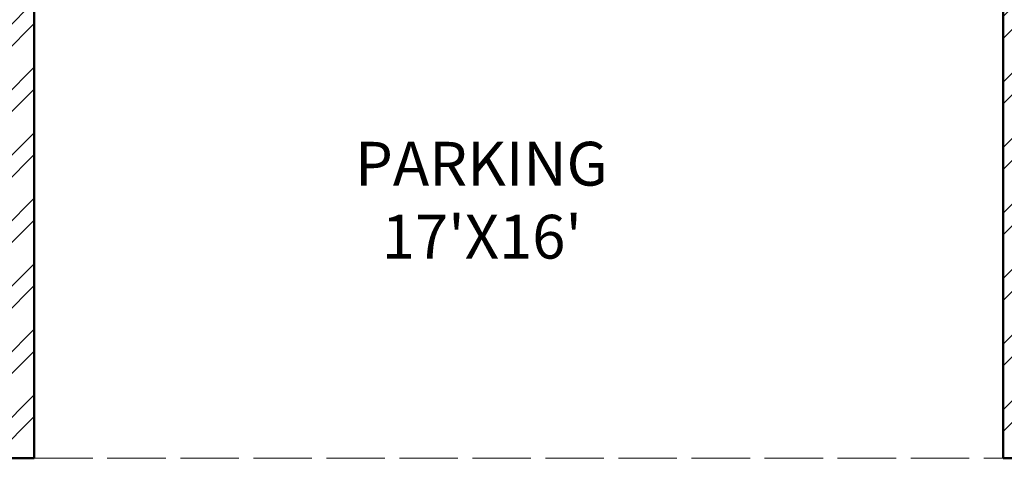
# Model space of a CAD drawing. Units: inches. Extents: x -31485 to -28799, y 18003 to 19130.
# Tile 2 of 15: x -30873 to -30670, y 18180 to 18270. Entities that reach past the tile are written whole.
import ezdxf

# ---------------------------------------------------------------- set-up
doc = ezdxf.new("R2010")
doc.units = ezdxf.units.IN
doc.linetypes.add('ACAD_ISO02W100', pattern=[15, 12, -3])
for name, color, linetype, lineweight in [('A-AREA-IDEN', 7, 'Continuous', 18), ('A-FLOR-OVHD', 30, 'ACAD_ISO02W100', 18), ('A-WALL', 7, 'Continuous', 50), ('A-WALL-PATT', 8, 'Continuous', 13)]:
    doc.layers.add(name, color=color, linetype=linetype, lineweight=lineweight)
doc.styles.get("Standard").update_dxf_attribs({"font": 'arial.ttf'})

msp = doc.modelspace()

# ---------------------------------------------------------------- hatches: boundary and pattern name
at = {"layer": 'A-WALL-PATT'}
h = msp.add_hatch(dxfattribs=at)
h.set_pattern_fill('ANSI32', color=256)
h.set_pattern_definition([(45, (-1687.357050595019, -0.3129728357926069), (-6.735192090801865, 6.735192090801866), []), (45, (-1682.866920595021, -0.3129728357926069), (-6.735192090801865, 6.735192090801866), [])])
h.paths.add_polyline_path([(-31156.52828769349, 18823.80296009311), (-31209.52828769349, 18823.80296009311), (-31209.52828769349, 18761.80296009311), (-31200.52828769349, 18761.80296009311), (-31200.52828769349, 18814.80296009311), (-31156.52828769349, 18814.80296009311)], flags=17)
h.paths.add_polyline_path([(-31022.5282876935, 18823.80296009311), (-31118.52828769349, 18823.80296009311), (-31118.52828769349, 18814.80296009311), (-31074.52828769349, 18814.80296009311), (-31074.52828769349, 18720.78574754094), (-31070.95696393926, 18720.78574754094), (-31068.52828769349, 18720.75952290947), (-31068.52828769349, 18814.80296009311), (-31022.5282876935, 18814.80296009311)], flags=17)
h.paths.add_polyline_path([(-30754.52828769349, 18823.80296009311), (-30850.5282876935, 18823.80296009311), (-30850.5282876935, 18814.80296009311), (-30806.5282876935, 18814.80296009311), (-30806.52828769349, 18723.10029278397), (-30800.5282876935, 18723.10029278397), (-30800.5282876935, 18814.80296009311), (-30754.52828769349, 18814.80296009311)], flags=17)
h.paths.add_polyline_path([(-30661.52828769349, 18823.80296009311), (-30716.52828769349, 18823.80296009311), (-30716.52828769349, 18814.80296009311), (-30670.52828769349, 18814.80296009311), (-30670.52828769349, 18761.80296009311), (-30661.52828769349, 18761.80296009311)], flags=17)
h.paths.add_polyline_path([(-30986.91891278487, 18670.80296009311), (-31068.52828769349, 18670.80296009311), (-31068.52828769349, 18684.75952290947), (-31074.52828769349, 18684.75952290947), (-31074.52828769349, 18670.80296009311), (-31200.52828769349, 18670.80296009311), (-31200.52828769349, 18723.80296009311), (-31209.52828769349, 18723.80296009311), (-31209.52828769349, 18641.80296009311), (-31200.52828769349, 18641.80296009311), (-31200.52828769349, 18664.80296009311), (-31104.52828769349, 18664.80296009311), (-31104.52828769349, 18628.92834044014), (-31098.52828769349, 18628.92834044014), (-31098.52828769348, 18664.8029600931), (-30986.91891278488, 18664.8029600931)], flags=17)
h.paths.add_polyline_path([(-30661.52828769349, 18723.80296009311), (-30670.52828769349, 18723.80296009311), (-30670.52828769349, 18670.80296009311), (-30800.5282876935, 18670.80296009311), (-30800.5282876935, 18687.10029278396), (-30806.52828769349, 18687.10029278396), (-30806.52828769349, 18670.80296009311), (-30885.59628027248, 18670.80296009311), (-30885.59628027248, 18667.80293426455), (-30885.59628027248, 18664.80296009311), (-30760.52828769349, 18664.80296009311), (-30760.52828769349, 18625.80296009311), (-30754.52828769349, 18625.80296009311), (-30754.52828769349, 18664.80296009311), (-30670.52828769349, 18664.80296009311), (-30670.52828769349, 18641.80296009311), (-30661.52828769349, 18641.80296009311)], flags=17)
h.paths.add_polyline_path([(-31200.52828769349, 18574.80296009311), (-31188.56436894977, 18574.80296009311), (-31188.56436894977, 18580.80296009311), (-31200.52828769349, 18580.80296009311), (-31200.52828769349, 18603.80296009311), (-31209.52828769349, 18603.80296009311), (-31209.52828769349, 18557.80296009311), (-31200.52828769349, 18557.80296009311)], flags=17)
h.paths.add_polyline_path([(-31098.52828769349, 18592.92834044014), (-31104.52828769349, 18592.92834044014), (-31104.52828769349, 18580.80296009311), (-31164.56436894977, 18580.80296009311), (-31164.56436894977, 18574.80296009311), (-31104.52828769349, 18574.80296009311), (-31104.52828769349, 18514.80296009311), (-31200.52828769349, 18514.80296009311), (-31200.52828769349, 18531.80296009311), (-31209.52828769349, 18531.80296009311), (-31209.52828769349, 18473.80296009311), (-31200.52828769349, 18473.80296009311), (-31200.52828769349, 18508.80296009311), (-31056.52828769349, 18508.80296009312), (-31056.52828769349, 18501.62307445529), (-31050.52828769349, 18501.62307445529), (-31050.52828769349, 18514.80296009311), (-31098.52828769349, 18514.80296009311)], flags=17)
h.paths.add_polyline_path([(-30661.52828769349, 18531.80296009311), (-30670.52828769349, 18531.80296009311), (-30670.52828769349, 18514.80296009311), (-30754.52828769349, 18514.80296009311), (-30754.52828769349, 18574.80296009311), (-30700.74522746605, 18574.80296009311), (-30700.74522746605, 18577.44024221289), (-30700.74522746605, 18580.8029600931), (-30754.52828769349, 18580.80296009311), (-30754.52828769349, 18589.80296009311), (-30760.52828769349, 18589.80296009311), (-30760.52828769349, 18514.80296009311), (-30820.52828769349, 18514.80296009311), (-30820.52828769348, 18499.26438911774), (-30814.52828769349, 18499.26438911774), (-30814.52828769349, 18508.80296009311), (-30670.52828769349, 18508.80296009311), (-30670.52828769349, 18473.80296009311), (-30661.52828769349, 18473.80296009311)], flags=17)
h.paths.add_polyline_path([(-30661.52828769349, 18435.80296009311), (-30670.52828769349, 18435.80296009311), (-30670.52828769349, 18400.80296009311), (-30814.52828769349, 18400.80296009311), (-30814.52828769349, 18413.15176302367), (-30820.52828769349, 18413.15176302367), (-30820.52828769349, 18400.80296009311), (-30932.52828769349, 18400.80296009311), (-30932.52828769349, 18664.80296009311), (-30921.59628027248, 18664.80296009311), (-30921.59628027248, 18670.80296009311), (-30932.5282876935, 18670.80296009311), (-30932.5282876935, 18814.80296009311), (-30888.5282876935, 18814.80296009311), (-30888.5282876935, 18823.80296009311), (-30984.5282876935, 18823.80296009311), (-30984.5282876935, 18814.80296009311), (-30938.5282876935, 18814.80296009311), (-30938.5282876935, 18670.80296009311), (-30950.91891278487, 18670.80296009311), (-30950.91891278488, 18664.80296009311), (-30938.5282876935, 18664.80296009311), (-30938.52828769349, 18400.80296009311), (-31050.52828769349, 18400.80296009311), (-31050.52828769349, 18411.18080736427), (-31056.52828769348, 18411.18080736427), (-31056.52828769348, 18400.80296009311), (-31200.52828769349, 18400.80296009311), (-31200.52828769349, 18435.80296009311), (-31209.52828769349, 18435.80296009311), (-31209.52828769349, 18179.80296009311), (-31200.52828769349, 18179.80296009311), (-31200.52828769349, 18394.80296009311), (-31001.52828769348, 18394.80296009311), (-31001.52828769348, 18179.80296009311), (-30954.52828769347, 18179.80296009311), (-30954.52828769347, 18188.80296009311), (-30995.52828769348, 18188.80296009311), (-30995.52828769348, 18394.80296009311), (-30875.52828769348, 18394.80296009311), (-30875.52828769348, 18188.80296009311), (-30916.52828769347, 18188.80296009311), (-30916.52828769347, 18179.80296009311), (-30869.52828769348, 18179.80296009311), (-30869.52828769348, 18394.80296009311), (-30670.52828769349, 18394.80296009311), (-30670.52828769349, 18179.80296009311), (-30661.52828769349, 18179.80296009311)])

# ---------------------------------------------------------------- linework, layer by layer
at = {"layer": 'A-FLOR-OVHD'}
msp.add_line((-30869.52828769348, 18179.80296009311), (-30670.52828769349, 18179.80296009311), dxfattribs=at)
at = {"layer": 'A-WALL'}
for p, q in [((-30869.52828769348, 18394.80296009311), (-30869.52828769348, 18179.80296009311)), ((-30670.52828769349, 18394.80296009311), (-30670.52828769349, 18179.80296009311)), ((-30869.52828769348, 18179.80296009311), (-31001.52828769348, 18179.80296009311)), ((-30661.52828769349, 18179.80296009311), (-30670.52828769349, 18179.80296009311))]:
    msp.add_line(p, q, dxfattribs=at)

# ---------------------------------------------------------------- texts
at = {"layer": 'A-AREA-IDEN', "insert": (-30803.65221329567, 18244.86089194873), "char_height": 9, "attachment_point": 1}
msp.add_mtext_dynamic_manual_height_columns("{PARKING\\P  17'X16'}", width=763.1478888985547, gutter_width=12.5, heights=[0], dxfattribs=at)

doc.saveas('drawing.dxf')
